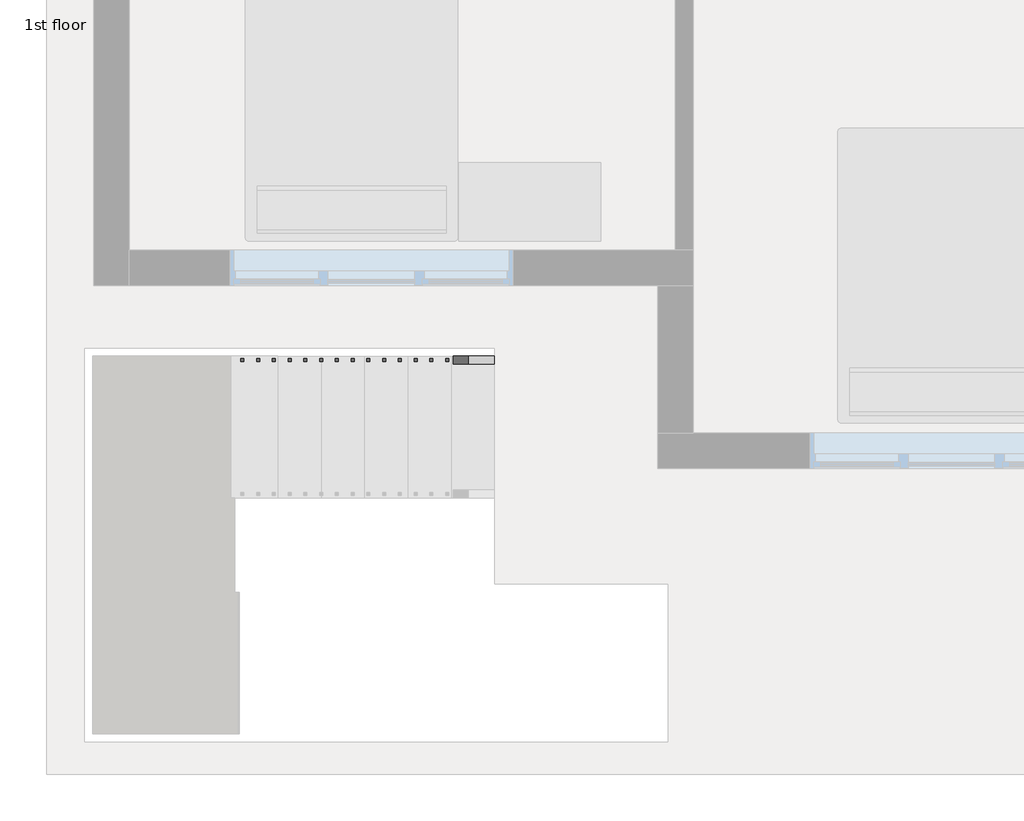
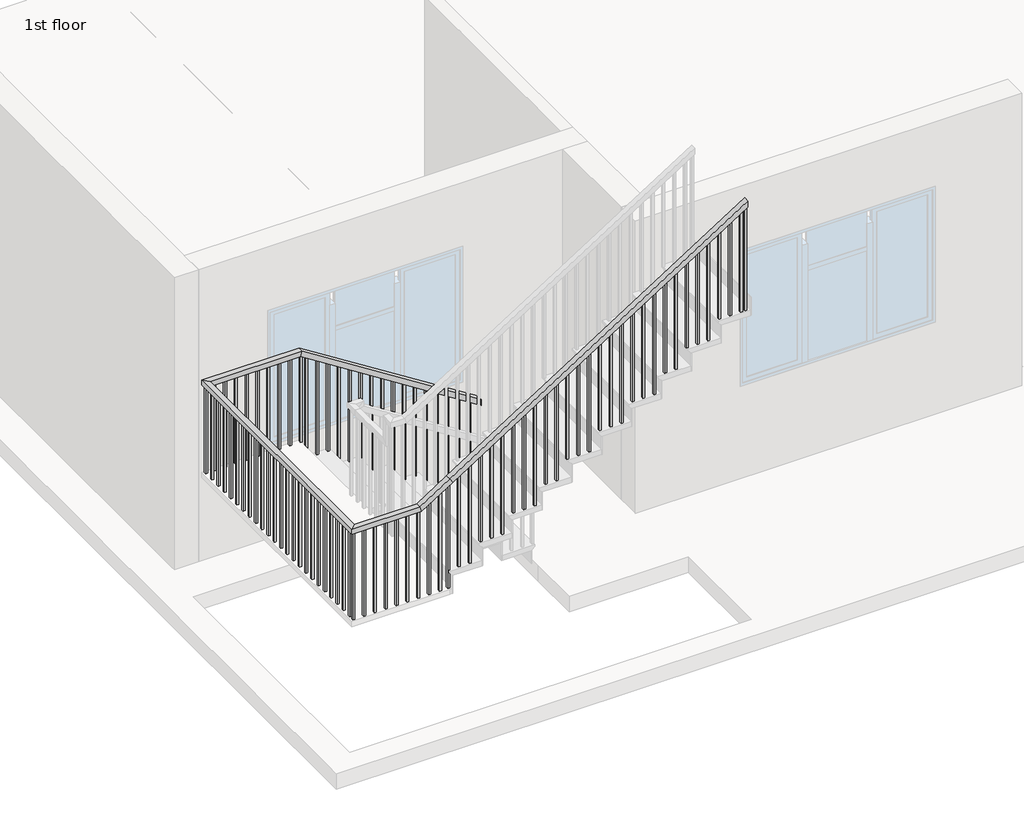
# One storey, part 3 of 4: 1 railing.
"""IFC4 building model written with IfcOpenShell, lengths in millimetres."""

from ifc_helpers import new_model, si_unit, frame, origin, place, context, project, spatial, polyline, outline, extrude, faceted_brep, element, save

model = new_model("IFC4")

# Units and contexts
model_context = context("Model", 3, world=origin())
ifc_project = project(units=[si_unit("LENGTHUNIT", "METRE", prefix="MILLI")], contexts=[model_context])

# Site, building, storey
site = spatial("IfcSite", under=ifc_project)
building = spatial("IfcBuilding", under=site)
storey = spatial("IfcBuildingStorey", under=building, Name="1st floor", Elevation=3810.0)

# Railing
placement = place(None, origin())
element("IfcRailing", 1, ObjectType="Handrail - Rectangular", at=placement, inside=storey, context=model_context, shape_type="SolidModel", body=[
    faceted_brep([(-6576.0763529, -1102.4338022, 4902.2), (-6576.0763529, -1102.4338022, 4841.986276), (-6576.0763529, -1051.6338022, 4841.986276), (-6576.0763529, -1051.6338022, 4902.2), (-8252.4763529, -1102.4338022, 5969.0), (-8267.2693478, -1102.4338022, 5918.2), (-8267.2693478, -1051.6338022, 5918.2), (-8252.4763529, -1051.6338022, 5969.0), (-9116.0763529, -1102.4338022, 5969.0), (-9116.0763529, -1102.4338022, 5918.2), (-9166.8763529, -1051.6338022, 5918.2), (-9166.8763529, -1051.6338022, 5969.0), (-9116.0763529, -3439.2338022, 5969.0), (-9116.0763529, -3439.2338022, 5918.2), (-9166.8763529, -3490.0338022, 5918.2), (-9166.8763529, -3490.0338022, 5969.0), (-8531.8763529, -3439.2338022, 5969.0), (-8517.083358, -3439.2338022, 5918.2), (-8517.083358, -3490.0338022, 5918.2), (-8531.8763529, -3490.0338022, 5969.0), (-8252.4763529, -3439.2338022, 6146.8), (-8225.2030779, -3439.2338022, 6103.9419964), (-8225.2030779, -3490.0338022, 6103.9419964), (-8252.4763529, -3490.0338022, 6146.8), (-5458.4763529, -3439.2338022, 7924.8), (-5458.4763529, -3490.0338022, 7924.8), (-5458.4763529, -3490.0338022, 7864.586276), (-5458.4763529, -3439.2338022, 7864.586276)], [[[0, 1, 2, 3]], [[1, 0, 4, 5]], [[2, 1, 5, 6]], [[3, 2, 6, 7]], [[0, 3, 7, 4]], [[5, 4, 8, 9]], [[6, 5, 9, 10]], [[7, 6, 10, 11]], [[4, 7, 11, 8]], [[9, 8, 12, 13]], [[10, 9, 13, 14]], [[11, 10, 14, 15]], [[8, 11, 15, 12]], [[13, 12, 16, 17]], [[14, 13, 17, 18]], [[15, 14, 18, 19]], [[12, 15, 19, 16]], [[17, 16, 20, 21]], [[18, 17, 21, 22]], [[19, 18, 22, 23]], [[16, 19, 23, 20]], [[24, 25, 26, 27]], [[21, 20, 24, 27]], [[22, 21, 27, 26]], [[23, 22, 26, 25]], [[20, 23, 25, 24]]]),
    extrude(outline(polyline([(7838.3203669, -5499.7513529), (7826.1976396, -5518.8013529), (6832.6, -5518.8013529), (6832.6, -5499.7513529), (7838.3203669, -5499.7513529)])), frame((0.0, -3474.1588022, 0.0), z_axis=(0.0, 1.0, 0.0), x_axis=(0.0, 0.0, 1.0)), (0.0, 0.0, 1.0), 19.05),
    extrude(outline(polyline([(7773.6658214, -5601.3513529), (7761.5430941, -5620.4013529), (6832.6, -5620.4013529), (6832.6, -5601.3513529), (7773.6658214, -5601.3513529)])), frame((0.0, -3474.1588022, 0.0), z_axis=(0.0, 1.0, 0.0), x_axis=(0.0, 0.0, 1.0)), (0.0, 0.0, 1.0), 19.05),
    extrude(outline(polyline([(7709.011276, -5702.9513529), (7696.8885487, -5722.0013529), (6832.6, -5722.0013529), (6832.6, -5702.9513529), (7709.011276, -5702.9513529)])), frame((0.0, -3474.1588022, 0.0), z_axis=(0.0, 1.0, 0.0), x_axis=(0.0, 0.0, 1.0)), (0.0, 0.0, 1.0), 19.05),
    extrude(outline(polyline([(7644.3567305, -5804.5513529), (7632.2340032, -5823.6013529), (6654.8, -5823.6013529), (6654.8, -5804.5513529), (7644.3567305, -5804.5513529)])), frame((0.0, -3474.1588022, 0.0), z_axis=(0.0, 1.0, 0.0), x_axis=(0.0, 0.0, 1.0)), (0.0, 0.0, 1.0), 19.05),
    extrude(outline(polyline([(7579.7021851, -5906.1513529), (7567.5794578, -5925.2013529), (6654.8, -5925.2013529), (6654.8, -5906.1513529), (7579.7021851, -5906.1513529)])), frame((0.0, -3474.1588022, 0.0), z_axis=(0.0, 1.0, 0.0), x_axis=(0.0, 0.0, 1.0)), (0.0, 0.0, 1.0), 19.05),
    extrude(outline(polyline([(7515.0476396, -6007.7513529), (7502.9249123, -6026.8013529), (6654.8, -6026.8013529), (6654.8, -6007.7513529), (7515.0476396, -6007.7513529)])), frame((0.0, -3474.1588022, 0.0), z_axis=(0.0, 1.0, 0.0), x_axis=(0.0, 0.0, 1.0)), (0.0, 0.0, 1.0), 19.05),
    extrude(outline(polyline([(7450.3930941, -6109.3513529), (7438.2703669, -6128.4013529), (6477.0, -6128.4013529), (6477.0, -6109.3513529), (7450.3930941, -6109.3513529)])), frame((0.0, -3474.1588022, 0.0), z_axis=(0.0, 1.0, 0.0), x_axis=(0.0, 0.0, 1.0)), (0.0, 0.0, 1.0), 19.05),
    extrude(outline(polyline([(7385.7385487, -6210.9513529), (7373.6158214, -6230.0013529), (6477.0, -6230.0013529), (6477.0, -6210.9513529), (7385.7385487, -6210.9513529)])), frame((0.0, -3474.1588022, 0.0), z_axis=(0.0, 1.0, 0.0), x_axis=(0.0, 0.0, 1.0)), (0.0, 0.0, 1.0), 19.05),
    extrude(outline(polyline([(7321.0840032, -6312.5513529), (7308.961276, -6331.6013529), (6299.2, -6331.6013529), (6299.2, -6312.5513529), (7321.0840032, -6312.5513529)])), frame((0.0, -3474.1588022, 0.0), z_axis=(0.0, 1.0, 0.0), x_axis=(0.0, 0.0, 1.0)), (0.0, 0.0, 1.0), 19.05),
    extrude(outline(polyline([(7256.4294578, -6414.1513529), (7244.3067305, -6433.2013529), (6299.2, -6433.2013529), (6299.2, -6414.1513529), (7256.4294578, -6414.1513529)])), frame((0.0, -3474.1588022, 0.0), z_axis=(0.0, 1.0, 0.0), x_axis=(0.0, 0.0, 1.0)), (0.0, 0.0, 1.0), 19.05),
    extrude(outline(polyline([(7191.7749123, -6515.7513529), (7179.6521851, -6534.8013529), (6299.2, -6534.8013529), (6299.2, -6515.7513529), (7191.7749123, -6515.7513529)])), frame((0.0, -3474.1588022, 0.0), z_axis=(0.0, 1.0, 0.0), x_axis=(0.0, 0.0, 1.0)), (0.0, 0.0, 1.0), 19.05),
    extrude(outline(polyline([(7127.1203669, -6617.3513529), (7114.9976396, -6636.4013529), (6121.4, -6636.4013529), (6121.4, -6617.3513529), (7127.1203669, -6617.3513529)])), frame((0.0, -3474.1588022, 0.0), z_axis=(0.0, 1.0, 0.0), x_axis=(0.0, 0.0, 1.0)), (0.0, 0.0, 1.0), 19.05),
    extrude(outline(polyline([(7062.4658214, -6718.9513529), (7050.3430941, -6738.0013529), (6121.4, -6738.0013529), (6121.4, -6718.9513529), (7062.4658214, -6718.9513529)])), frame((0.0, -3474.1588022, 0.0), z_axis=(0.0, 1.0, 0.0), x_axis=(0.0, 0.0, 1.0)), (0.0, 0.0, 1.0), 19.05),
    extrude(outline(polyline([(6997.811276, -6820.5513529), (6985.6885487, -6839.6013529), (6121.4, -6839.6013529), (6121.4, -6820.5513529), (6997.811276, -6820.5513529)])), frame((0.0, -3474.1588022, 0.0), z_axis=(0.0, 1.0, 0.0), x_axis=(0.0, 0.0, 1.0)), (0.0, 0.0, 1.0), 19.05),
    extrude(outline(polyline([(6933.1567305, -6922.1513529), (6921.0340032, -6941.2013529), (5943.6, -6941.2013529), (5943.6, -6922.1513529), (6933.1567305, -6922.1513529)])), frame((0.0, -3474.1588022, 0.0), z_axis=(0.0, 1.0, 0.0), x_axis=(0.0, 0.0, 1.0)), (0.0, 0.0, 1.0), 19.05),
    extrude(outline(polyline([(6868.5021851, -7023.7513529), (6856.3794578, -7042.8013529), (5943.6, -7042.8013529), (5943.6, -7023.7513529), (6868.5021851, -7023.7513529)])), frame((0.0, -3474.1588022, 0.0), z_axis=(0.0, 1.0, 0.0), x_axis=(0.0, 0.0, 1.0)), (0.0, 0.0, 1.0), 19.05),
    extrude(outline(polyline([(6803.8476396, -7125.3513529), (6791.7249123, -7144.4013529), (5943.6, -7144.4013529), (5943.6, -7125.3513529), (6803.8476396, -7125.3513529)])), frame((0.0, -3474.1588022, 0.0), z_axis=(0.0, 1.0, 0.0), x_axis=(0.0, 0.0, 1.0)), (0.0, 0.0, 1.0), 19.05),
    extrude(outline(polyline([(6739.1930941, -7226.9513529), (6727.0703669, -7246.0013529), (5765.8, -7246.0013529), (5765.8, -7226.9513529), (6739.1930941, -7226.9513529)])), frame((0.0, -3474.1588022, 0.0), z_axis=(0.0, 1.0, 0.0), x_axis=(0.0, 0.0, 1.0)), (0.0, 0.0, 1.0), 19.05),
    extrude(outline(polyline([(6674.5385487, -7328.5513529), (6662.4158214, -7347.6013529), (5765.8, -7347.6013529), (5765.8, -7328.5513529), (6674.5385487, -7328.5513529)])), frame((0.0, -3474.1588022, 0.0), z_axis=(0.0, 1.0, 0.0), x_axis=(0.0, 0.0, 1.0)), (0.0, 0.0, 1.0), 19.05),
    extrude(outline(polyline([(6609.8840032, -7430.1513529), (6597.761276, -7449.2013529), (5588.0, -7449.2013529), (5588.0, -7430.1513529), (6609.8840032, -7430.1513529)])), frame((0.0, -3474.1588022, 0.0), z_axis=(0.0, 1.0, 0.0), x_axis=(0.0, 0.0, 1.0)), (0.0, 0.0, 1.0), 19.05),
    extrude(outline(polyline([(6545.2294578, -7531.7513529), (6533.1067305, -7550.8013529), (5588.0, -7550.8013529), (5588.0, -7531.7513529), (6545.2294578, -7531.7513529)])), frame((0.0, -3474.1588022, 0.0), z_axis=(0.0, 1.0, 0.0), x_axis=(0.0, 0.0, 1.0)), (0.0, 0.0, 1.0), 19.05),
    extrude(outline(polyline([(6480.5749123, -7633.3513529), (6468.4521851, -7652.4013529), (5588.0, -7652.4013529), (5588.0, -7633.3513529), (6480.5749123, -7633.3513529)])), frame((0.0, -3474.1588022, 0.0), z_axis=(0.0, 1.0, 0.0), x_axis=(0.0, 0.0, 1.0)), (0.0, 0.0, 1.0), 19.05),
    extrude(outline(polyline([(6415.9203669, -7734.9513529), (6403.7976396, -7754.0013529), (5410.2, -7754.0013529), (5410.2, -7734.9513529), (6415.9203669, -7734.9513529)])), frame((0.0, -3474.1588022, 0.0), z_axis=(0.0, 1.0, 0.0), x_axis=(0.0, 0.0, 1.0)), (0.0, 0.0, 1.0), 19.05),
    extrude(outline(polyline([(6351.2658214, -7836.5513529), (6339.1430941, -7855.6013529), (5410.2, -7855.6013529), (5410.2, -7836.5513529), (6351.2658214, -7836.5513529)])), frame((0.0, -3474.1588022, 0.0), z_axis=(0.0, 1.0, 0.0), x_axis=(0.0, 0.0, 1.0)), (0.0, 0.0, 1.0), 19.05),
    extrude(outline(polyline([(6286.611276, -7938.1513529), (6274.4885487, -7957.2013529), (5410.2, -7957.2013529), (5410.2, -7938.1513529), (6286.611276, -7938.1513529)])), frame((0.0, -3474.1588022, 0.0), z_axis=(0.0, 1.0, 0.0), x_axis=(0.0, 0.0, 1.0)), (0.0, 0.0, 1.0), 19.05),
    extrude(outline(polyline([(6221.9567305, -8039.7513529), (6209.8340032, -8058.8013529), (5232.4, -8058.8013529), (5232.4, -8039.7513529), (6221.9567305, -8039.7513529)])), frame((0.0, -3474.1588022, 0.0), z_axis=(0.0, 1.0, 0.0), x_axis=(0.0, 0.0, 1.0)), (0.0, 0.0, 1.0), 19.05),
    extrude(outline(polyline([(6157.3021851, -8141.3513529), (6145.1794578, -8160.4013529), (5232.4, -8160.4013529), (5232.4, -8141.3513529), (6157.3021851, -8141.3513529)])), frame((0.0, -3474.1588022, 0.0), z_axis=(0.0, 1.0, 0.0), x_axis=(0.0, 0.0, 1.0)), (0.0, 0.0, 1.0), 19.05),
    extrude(outline(polyline([(6044.1567305, -8319.1513529), (6032.0340032, -8338.2013529), (5054.6, -8338.2013529), (5054.6, -8319.1513529), (6044.1567305, -8319.1513529)])), frame((0.0, -3474.1588022, 0.0), z_axis=(0.0, 1.0, 0.0), x_axis=(0.0, 0.0, 1.0)), (0.0, 0.0, 1.0), 19.05),
    extrude(outline(polyline([(5979.5021851, -8420.7513529), (5967.3794578, -8439.8013529), (5054.6, -8439.8013529), (5054.6, -8420.7513529), (5979.5021851, -8420.7513529)])), frame((0.0, -3474.1588022, 0.0), z_axis=(0.0, 1.0, 0.0), x_axis=(0.0, 0.0, 1.0)), (0.0, 0.0, 1.0), 19.05),
    extrude(outline(polyline([(-8541.4013529, -3474.1588022), (-8541.4013529, -3455.1088022), (-8522.3513529, -3455.1088022), (-8522.3513529, -3474.1588022), (-8541.4013529, -3474.1588022)])), frame((0.0, 0.0, 5054.6), z_axis=(0.0, 0.0, 1.0), x_axis=(1.0, 0.0, 0.0)), (0.0, 0.0, 1.0), 863.6),
    extrude(outline(polyline([(-8643.0013529, -3474.1588022), (-8643.0013529, -3455.1088022), (-8623.9513529, -3455.1088022), (-8623.9513529, -3474.1588022), (-8643.0013529, -3474.1588022)])), frame((0.0, 0.0, 5054.6), z_axis=(0.0, 0.0, 1.0), x_axis=(1.0, 0.0, 0.0)), (0.0, 0.0, 1.0), 863.6),
    extrude(outline(polyline([(-8744.6013529, -3474.1588022), (-8744.6013529, -3455.1088022), (-8725.5513529, -3455.1088022), (-8725.5513529, -3474.1588022), (-8744.6013529, -3474.1588022)])), frame((0.0, 0.0, 5054.6), z_axis=(0.0, 0.0, 1.0), x_axis=(1.0, 0.0, 0.0)), (0.0, 0.0, 1.0), 863.6),
    extrude(outline(polyline([(-8846.2013529, -3474.1588022), (-8846.2013529, -3455.1088022), (-8827.1513529, -3455.1088022), (-8827.1513529, -3474.1588022), (-8846.2013529, -3474.1588022)])), frame((0.0, 0.0, 5054.6), z_axis=(0.0, 0.0, 1.0), x_axis=(1.0, 0.0, 0.0)), (0.0, 0.0, 1.0), 863.6),
    extrude(outline(polyline([(-8947.8013529, -3474.1588022), (-8947.8013529, -3455.1088022), (-8928.7513529, -3455.1088022), (-8928.7513529, -3474.1588022), (-8947.8013529, -3474.1588022)])), frame((0.0, 0.0, 5054.6), z_axis=(0.0, 0.0, 1.0), x_axis=(1.0, 0.0, 0.0)), (0.0, 0.0, 1.0), 863.6),
    extrude(outline(polyline([(-9049.4013529, -3474.1588022), (-9049.4013529, -3455.1088022), (-9030.3513529, -3455.1088022), (-9030.3513529, -3474.1588022), (-9049.4013529, -3474.1588022)])), frame((0.0, 0.0, 5054.6), z_axis=(0.0, 0.0, 1.0), x_axis=(1.0, 0.0, 0.0)), (0.0, 0.0, 1.0), 863.6),
    extrude(outline(polyline([(-9151.0013529, -3404.3088022), (-9131.9513529, -3404.3088022), (-9131.9513529, -3423.3588022), (-9151.0013529, -3423.3588022), (-9151.0013529, -3404.3088022)])), frame((0.0, 0.0, 5054.6), z_axis=(0.0, 0.0, 1.0), x_axis=(1.0, 0.0, 0.0)), (0.0, 0.0, 1.0), 863.6),
    extrude(outline(polyline([(-9151.0013529, -3302.7088022), (-9131.9513529, -3302.7088022), (-9131.9513529, -3321.7588022), (-9151.0013529, -3321.7588022), (-9151.0013529, -3302.7088022)])), frame((0.0, 0.0, 5054.6), z_axis=(0.0, 0.0, 1.0), x_axis=(1.0, 0.0, 0.0)), (0.0, 0.0, 1.0), 863.6),
    extrude(outline(polyline([(-9151.0013529, -3201.1088022), (-9131.9513529, -3201.1088022), (-9131.9513529, -3220.1588022), (-9151.0013529, -3220.1588022), (-9151.0013529, -3201.1088022)])), frame((0.0, 0.0, 5054.6), z_axis=(0.0, 0.0, 1.0), x_axis=(1.0, 0.0, 0.0)), (0.0, 0.0, 1.0), 863.6),
    extrude(outline(polyline([(-9151.0013529, -3099.5088022), (-9131.9513529, -3099.5088022), (-9131.9513529, -3118.5588022), (-9151.0013529, -3118.5588022), (-9151.0013529, -3099.5088022)])), frame((0.0, 0.0, 5054.6), z_axis=(0.0, 0.0, 1.0), x_axis=(1.0, 0.0, 0.0)), (0.0, 0.0, 1.0), 863.6),
    extrude(outline(polyline([(-9151.0013529, -2997.9088022), (-9131.9513529, -2997.9088022), (-9131.9513529, -3016.9588022), (-9151.0013529, -3016.9588022), (-9151.0013529, -2997.9088022)])), frame((0.0, 0.0, 5054.6), z_axis=(0.0, 0.0, 1.0), x_axis=(1.0, 0.0, 0.0)), (0.0, 0.0, 1.0), 863.6),
    extrude(outline(polyline([(-9151.0013529, -2896.3088022), (-9131.9513529, -2896.3088022), (-9131.9513529, -2915.3588022), (-9151.0013529, -2915.3588022), (-9151.0013529, -2896.3088022)])), frame((0.0, 0.0, 5054.6), z_axis=(0.0, 0.0, 1.0), x_axis=(1.0, 0.0, 0.0)), (0.0, 0.0, 1.0), 863.6),
    extrude(outline(polyline([(-9151.0013529, -2794.7088022), (-9131.9513529, -2794.7088022), (-9131.9513529, -2813.7588022), (-9151.0013529, -2813.7588022), (-9151.0013529, -2794.7088022)])), frame((0.0, 0.0, 5054.6), z_axis=(0.0, 0.0, 1.0), x_axis=(1.0, 0.0, 0.0)), (0.0, 0.0, 1.0), 863.6),
    extrude(outline(polyline([(-9151.0013529, -2693.1088022), (-9131.9513529, -2693.1088022), (-9131.9513529, -2712.1588022), (-9151.0013529, -2712.1588022), (-9151.0013529, -2693.1088022)])), frame((0.0, 0.0, 5054.6), z_axis=(0.0, 0.0, 1.0), x_axis=(1.0, 0.0, 0.0)), (0.0, 0.0, 1.0), 863.6),
    extrude(outline(polyline([(-9151.0013529, -2591.5088022), (-9131.9513529, -2591.5088022), (-9131.9513529, -2610.5588022), (-9151.0013529, -2610.5588022), (-9151.0013529, -2591.5088022)])), frame((0.0, 0.0, 5054.6), z_axis=(0.0, 0.0, 1.0), x_axis=(1.0, 0.0, 0.0)), (0.0, 0.0, 1.0), 863.6),
    extrude(outline(polyline([(-9151.0013529, -2489.9088022), (-9131.9513529, -2489.9088022), (-9131.9513529, -2508.9588022), (-9151.0013529, -2508.9588022), (-9151.0013529, -2489.9088022)])), frame((0.0, 0.0, 5054.6), z_axis=(0.0, 0.0, 1.0), x_axis=(1.0, 0.0, 0.0)), (0.0, 0.0, 1.0), 863.6),
    extrude(outline(polyline([(-9151.0013529, -2388.3088022), (-9131.9513529, -2388.3088022), (-9131.9513529, -2407.3588022), (-9151.0013529, -2407.3588022), (-9151.0013529, -2388.3088022)])), frame((0.0, 0.0, 5054.6), z_axis=(0.0, 0.0, 1.0), x_axis=(1.0, 0.0, 0.0)), (0.0, 0.0, 1.0), 863.6),
    extrude(outline(polyline([(-9151.0013529, -2286.7088022), (-9131.9513529, -2286.7088022), (-9131.9513529, -2305.7588022), (-9151.0013529, -2305.7588022), (-9151.0013529, -2286.7088022)])), frame((0.0, 0.0, 5054.6), z_axis=(0.0, 0.0, 1.0), x_axis=(1.0, 0.0, 0.0)), (0.0, 0.0, 1.0), 863.6),
    extrude(outline(polyline([(-9151.0013529, -2185.1088022), (-9131.9513529, -2185.1088022), (-9131.9513529, -2204.1588022), (-9151.0013529, -2204.1588022), (-9151.0013529, -2185.1088022)])), frame((0.0, 0.0, 5054.6), z_axis=(0.0, 0.0, 1.0), x_axis=(1.0, 0.0, 0.0)), (0.0, 0.0, 1.0), 863.6),
    extrude(outline(polyline([(-9151.0013529, -2083.5088022), (-9131.9513529, -2083.5088022), (-9131.9513529, -2102.5588022), (-9151.0013529, -2102.5588022), (-9151.0013529, -2083.5088022)])), frame((0.0, 0.0, 5054.6), z_axis=(0.0, 0.0, 1.0), x_axis=(1.0, 0.0, 0.0)), (0.0, 0.0, 1.0), 863.6),
    extrude(outline(polyline([(-9151.0013529, -1981.9088022), (-9131.9513529, -1981.9088022), (-9131.9513529, -2000.9588022), (-9151.0013529, -2000.9588022), (-9151.0013529, -1981.9088022)])), frame((0.0, 0.0, 5054.6), z_axis=(0.0, 0.0, 1.0), x_axis=(1.0, 0.0, 0.0)), (0.0, 0.0, 1.0), 863.6),
    extrude(outline(polyline([(-9151.0013529, -1880.3088022), (-9131.9513529, -1880.3088022), (-9131.9513529, -1899.3588022), (-9151.0013529, -1899.3588022), (-9151.0013529, -1880.3088022)])), frame((0.0, 0.0, 5054.6), z_axis=(0.0, 0.0, 1.0), x_axis=(1.0, 0.0, 0.0)), (0.0, 0.0, 1.0), 863.6),
    extrude(outline(polyline([(-9151.0013529, -1778.7088022), (-9131.9513529, -1778.7088022), (-9131.9513529, -1797.7588022), (-9151.0013529, -1797.7588022), (-9151.0013529, -1778.7088022)])), frame((0.0, 0.0, 5054.6), z_axis=(0.0, 0.0, 1.0), x_axis=(1.0, 0.0, 0.0)), (0.0, 0.0, 1.0), 863.6),
    extrude(outline(polyline([(-9151.0013529, -1677.1088022), (-9131.9513529, -1677.1088022), (-9131.9513529, -1696.1588022), (-9151.0013529, -1696.1588022), (-9151.0013529, -1677.1088022)])), frame((0.0, 0.0, 5054.6), z_axis=(0.0, 0.0, 1.0), x_axis=(1.0, 0.0, 0.0)), (0.0, 0.0, 1.0), 863.6),
    extrude(outline(polyline([(-9151.0013529, -1575.5088022), (-9131.9513529, -1575.5088022), (-9131.9513529, -1594.5588022), (-9151.0013529, -1594.5588022), (-9151.0013529, -1575.5088022)])), frame((0.0, 0.0, 5054.6), z_axis=(0.0, 0.0, 1.0), x_axis=(1.0, 0.0, 0.0)), (0.0, 0.0, 1.0), 863.6),
    extrude(outline(polyline([(-9151.0013529, -1473.9088022), (-9131.9513529, -1473.9088022), (-9131.9513529, -1492.9588022), (-9151.0013529, -1492.9588022), (-9151.0013529, -1473.9088022)])), frame((0.0, 0.0, 5054.6), z_axis=(0.0, 0.0, 1.0), x_axis=(1.0, 0.0, 0.0)), (0.0, 0.0, 1.0), 863.6),
    extrude(outline(polyline([(-9151.0013529, -1372.3088022), (-9131.9513529, -1372.3088022), (-9131.9513529, -1391.3588022), (-9151.0013529, -1391.3588022), (-9151.0013529, -1372.3088022)])), frame((0.0, 0.0, 5054.6), z_axis=(0.0, 0.0, 1.0), x_axis=(1.0, 0.0, 0.0)), (0.0, 0.0, 1.0), 863.6),
    extrude(outline(polyline([(-9151.0013529, -1270.7088022), (-9131.9513529, -1270.7088022), (-9131.9513529, -1289.7588022), (-9151.0013529, -1289.7588022), (-9151.0013529, -1270.7088022)])), frame((0.0, 0.0, 5054.6), z_axis=(0.0, 0.0, 1.0), x_axis=(1.0, 0.0, 0.0)), (0.0, 0.0, 1.0), 863.6),
    extrude(outline(polyline([(-9151.0013529, -1169.1088022), (-9131.9513529, -1169.1088022), (-9131.9513529, -1188.1588022), (-9151.0013529, -1188.1588022), (-9151.0013529, -1169.1088022)])), frame((0.0, 0.0, 5054.6), z_axis=(0.0, 0.0, 1.0), x_axis=(1.0, 0.0, 0.0)), (0.0, 0.0, 1.0), 863.6),
    extrude(outline(polyline([(-9055.7513529, -1067.5088022), (-9055.7513529, -1086.5588022), (-9074.8013529, -1086.5588022), (-9074.8013529, -1067.5088022), (-9055.7513529, -1067.5088022)])), frame((0.0, 0.0, 5054.6), z_axis=(0.0, 0.0, 1.0), x_axis=(1.0, 0.0, 0.0)), (0.0, 0.0, 1.0), 863.6),
    extrude(outline(polyline([(-8954.1513529, -1067.5088022), (-8954.1513529, -1086.5588022), (-8973.2013529, -1086.5588022), (-8973.2013529, -1067.5088022), (-8954.1513529, -1067.5088022)])), frame((0.0, 0.0, 5054.6), z_axis=(0.0, 0.0, 1.0), x_axis=(1.0, 0.0, 0.0)), (0.0, 0.0, 1.0), 863.6),
    extrude(outline(polyline([(-8852.5513529, -1067.5088022), (-8852.5513529, -1086.5588022), (-8871.6013529, -1086.5588022), (-8871.6013529, -1067.5088022), (-8852.5513529, -1067.5088022)])), frame((0.0, 0.0, 5054.6), z_axis=(0.0, 0.0, 1.0), x_axis=(1.0, 0.0, 0.0)), (0.0, 0.0, 1.0), 863.6),
    extrude(outline(polyline([(-8750.9513529, -1067.5088022), (-8750.9513529, -1086.5588022), (-8770.0013529, -1086.5588022), (-8770.0013529, -1067.5088022), (-8750.9513529, -1067.5088022)])), frame((0.0, 0.0, 5054.6), z_axis=(0.0, 0.0, 1.0), x_axis=(1.0, 0.0, 0.0)), (0.0, 0.0, 1.0), 863.6),
    extrude(outline(polyline([(-8649.3513529, -1067.5088022), (-8649.3513529, -1086.5588022), (-8668.4013529, -1086.5588022), (-8668.4013529, -1067.5088022), (-8649.3513529, -1067.5088022)])), frame((0.0, 0.0, 5054.6), z_axis=(0.0, 0.0, 1.0), x_axis=(1.0, 0.0, 0.0)), (0.0, 0.0, 1.0), 863.6),
    extrude(outline(polyline([(-8547.7513529, -1067.5088022), (-8547.7513529, -1086.5588022), (-8566.8013529, -1086.5588022), (-8566.8013529, -1067.5088022), (-8547.7513529, -1067.5088022)])), frame((0.0, 0.0, 5054.6), z_axis=(0.0, 0.0, 1.0), x_axis=(1.0, 0.0, 0.0)), (0.0, 0.0, 1.0), 863.6),
    extrude(outline(polyline([(-8446.1513529, -1067.5088022), (-8446.1513529, -1086.5588022), (-8465.2013529, -1086.5588022), (-8465.2013529, -1067.5088022), (-8446.1513529, -1067.5088022)])), frame((0.0, 0.0, 5054.6), z_axis=(0.0, 0.0, 1.0), x_axis=(1.0, 0.0, 0.0)), (0.0, 0.0, 1.0), 863.6),
    extrude(outline(polyline([(-8344.5513529, -1067.5088022), (-8344.5513529, -1086.5588022), (-8363.6013529, -1086.5588022), (-8363.6013529, -1067.5088022), (-8344.5513529, -1067.5088022)])), frame((0.0, 0.0, 5054.6), z_axis=(0.0, 0.0, 1.0), x_axis=(1.0, 0.0, 0.0)), (0.0, 0.0, 1.0), 863.6),
    extrude(outline(polyline([(5870.3976396, -8192.1513529), (5882.5203669, -8211.2013529), (4876.8, -8211.2013529), (4876.8, -8192.1513529), (5870.3976396, -8192.1513529)])), frame((0.0, -1086.5588022, 0.0), z_axis=(0.0, 1.0, 0.0), x_axis=(0.0, 0.0, 1.0)), (0.0, 0.0, 1.0), 19.05),
    extrude(outline(polyline([(5805.7430941, -8090.5513529), (5817.8658214, -8109.6013529), (4876.8, -8109.6013529), (4876.8, -8090.5513529), (5805.7430941, -8090.5513529)])), frame((0.0, -1086.5588022, 0.0), z_axis=(0.0, 1.0, 0.0), x_axis=(0.0, 0.0, 1.0)), (0.0, 0.0, 1.0), 19.05),
    extrude(outline(polyline([(5741.0885487, -7988.9513529), (5753.211276, -8008.0013529), (4876.8, -8008.0013529), (4876.8, -7988.9513529), (5741.0885487, -7988.9513529)])), frame((0.0, -1086.5588022, 0.0), z_axis=(0.0, 1.0, 0.0), x_axis=(0.0, 0.0, 1.0)), (0.0, 0.0, 1.0), 19.05),
    extrude(outline(polyline([(5676.4340032, -7887.3513529), (5688.5567305, -7906.4013529), (4699.0, -7906.4013529), (4699.0, -7887.3513529), (5676.4340032, -7887.3513529)])), frame((0.0, -1086.5588022, 0.0), z_axis=(0.0, 1.0, 0.0), x_axis=(0.0, 0.0, 1.0)), (0.0, 0.0, 1.0), 19.05),
    extrude(outline(polyline([(5611.7794578, -7785.7513529), (5623.9021851, -7804.8013529), (4699.0, -7804.8013529), (4699.0, -7785.7513529), (5611.7794578, -7785.7513529)])), frame((0.0, -1086.5588022, 0.0), z_axis=(0.0, 1.0, 0.0), x_axis=(0.0, 0.0, 1.0)), (0.0, 0.0, 1.0), 19.05),
    extrude(outline(polyline([(5547.1249123, -7684.1513529), (5559.2476396, -7703.2013529), (4699.0, -7703.2013529), (4699.0, -7684.1513529), (5547.1249123, -7684.1513529)])), frame((0.0, -1086.5588022, 0.0), z_axis=(0.0, 1.0, 0.0), x_axis=(0.0, 0.0, 1.0)), (0.0, 0.0, 1.0), 19.05),
    extrude(outline(polyline([(5482.4703669, -7582.5513529), (5494.5930941, -7601.6013529), (4521.2, -7601.6013529), (4521.2, -7582.5513529), (5482.4703669, -7582.5513529)])), frame((0.0, -1086.5588022, 0.0), z_axis=(0.0, 1.0, 0.0), x_axis=(0.0, 0.0, 1.0)), (0.0, 0.0, 1.0), 19.05),
    extrude(outline(polyline([(5417.8158214, -7480.9513529), (5429.9385487, -7500.0013529), (4521.2, -7500.0013529), (4521.2, -7480.9513529), (5417.8158214, -7480.9513529)])), frame((0.0, -1086.5588022, 0.0), z_axis=(0.0, 1.0, 0.0), x_axis=(0.0, 0.0, 1.0)), (0.0, 0.0, 1.0), 19.05),
    extrude(outline(polyline([(5353.161276, -7379.3513529), (5365.2840032, -7398.4013529), (4343.4, -7398.4013529), (4343.4, -7379.3513529), (5353.161276, -7379.3513529)])), frame((0.0, -1086.5588022, 0.0), z_axis=(0.0, 1.0, 0.0), x_axis=(0.0, 0.0, 1.0)), (0.0, 0.0, 1.0), 19.05),
    extrude(outline(polyline([(5288.5067305, -7277.7513529), (5300.6294578, -7296.8013529), (4343.4, -7296.8013529), (4343.4, -7277.7513529), (5288.5067305, -7277.7513529)])), frame((0.0, -1086.5588022, 0.0), z_axis=(0.0, 1.0, 0.0), x_axis=(0.0, 0.0, 1.0)), (0.0, 0.0, 1.0), 19.05),
    extrude(outline(polyline([(5223.8521851, -7176.1513529), (5235.9749123, -7195.2013529), (4343.4, -7195.2013529), (4343.4, -7176.1513529), (5223.8521851, -7176.1513529)])), frame((0.0, -1086.5588022, 0.0), z_axis=(0.0, 1.0, 0.0), x_axis=(0.0, 0.0, 1.0)), (0.0, 0.0, 1.0), 19.05),
    extrude(outline(polyline([(5159.1976396, -7074.5513529), (5171.3203669, -7093.6013529), (4165.6, -7093.6013529), (4165.6, -7074.5513529), (5159.1976396, -7074.5513529)])), frame((0.0, -1086.5588022, 0.0), z_axis=(0.0, 1.0, 0.0), x_axis=(0.0, 0.0, 1.0)), (0.0, 0.0, 1.0), 19.05),
    extrude(outline(polyline([(5094.5430941, -6972.9513529), (5106.6658214, -6992.0013529), (4165.6, -6992.0013529), (4165.6, -6972.9513529), (5094.5430941, -6972.9513529)])), frame((0.0, -1086.5588022, 0.0), z_axis=(0.0, 1.0, 0.0), x_axis=(0.0, 0.0, 1.0)), (0.0, 0.0, 1.0), 19.05),
    extrude(outline(polyline([(5029.8885487, -6871.3513529), (5042.011276, -6890.4013529), (4165.6, -6890.4013529), (4165.6, -6871.3513529), (5029.8885487, -6871.3513529)])), frame((0.0, -1086.5588022, 0.0), z_axis=(0.0, 1.0, 0.0), x_axis=(0.0, 0.0, 1.0)), (0.0, 0.0, 1.0), 19.05),
    extrude(outline(polyline([(4965.2340032, -6769.7513529), (4977.3567305, -6788.8013529), (3987.8, -6788.8013529), (3987.8, -6769.7513529), (4965.2340032, -6769.7513529)])), frame((0.0, -1086.5588022, 0.0), z_axis=(0.0, 1.0, 0.0), x_axis=(0.0, 0.0, 1.0)), (0.0, 0.0, 1.0), 19.05),
    extrude(outline(polyline([(4900.5794578, -6668.1513529), (4912.7021851, -6687.2013529), (3987.8, -6687.2013529), (3987.8, -6668.1513529), (4900.5794578, -6668.1513529)])), frame((0.0, -1086.5588022, 0.0), z_axis=(0.0, 1.0, 0.0), x_axis=(0.0, 0.0, 1.0)), (0.0, 0.0, 1.0), 19.05),
    extrude(outline(polyline([(6092.6476396, -8242.9513529), (6080.5249123, -8262.0013529), (5054.6, -8262.0013529), (5054.6, -8242.9513529), (6092.6476396, -8242.9513529)])), frame((0.0, -3474.1588022, 0.0), z_axis=(0.0, 1.0, 0.0), x_axis=(0.0, 0.0, 1.0)), (0.0, 0.0, 1.0), 19.05),
    extrude(outline(polyline([(-9151.0013529, -3455.1088022), (-9131.9513529, -3455.1088022), (-9131.9513529, -3474.1588022), (-9151.0013529, -3474.1588022), (-9151.0013529, -3455.1088022)])), frame((0.0, 0.0, 5054.6), z_axis=(0.0, 0.0, 1.0), x_axis=(1.0, 0.0, 0.0)), (0.0, 0.0, 1.0), 863.6),
    extrude(outline(polyline([(-9131.9513529, -1067.5088022), (-9131.9513529, -1086.5588022), (-9151.0013529, -1086.5588022), (-9151.0013529, -1067.5088022), (-9131.9513529, -1067.5088022)])), frame((0.0, 0.0, 5054.6), z_axis=(0.0, 0.0, 1.0), x_axis=(1.0, 0.0, 0.0)), (0.0, 0.0, 1.0), 863.6),
    extrude(outline(polyline([(5902.7249123, -8242.9513529), (5914.8476396, -8262.0013529), (5054.6, -8262.0013529), (5054.6, -8242.9513529), (5902.7249123, -8242.9513529)])), frame((0.0, -1086.5588022, 0.0), z_axis=(0.0, 1.0, 0.0), x_axis=(0.0, 0.0, 1.0)), (0.0, 0.0, 1.0), 19.05),
    extrude(outline(polyline([(7864.586276, -5458.4763529), (7852.4635487, -5477.5263529), (6832.6, -5477.5263529), (6832.6, -5458.4763529), (7864.586276, -5458.4763529)])), frame((0.0, -3474.1588022, 0.0), z_axis=(0.0, 1.0, 0.0), x_axis=(0.0, 0.0, 1.0)), (0.0, 0.0, 1.0), 19.05),
    extrude(outline(polyline([(4841.986276, -6576.0763529), (4854.1090032, -6595.1263529), (3987.8, -6595.1263529), (3987.8, -6576.0763529), (4841.986276, -6576.0763529)])), frame((0.0, -1086.5588022, 0.0), z_axis=(0.0, 1.0, 0.0), x_axis=(0.0, 0.0, 1.0)), (0.0, 0.0, 1.0), 19.05),
])

save(model, "model.ifc")

# Revit data of these elements
# Type "Handrail - Rectangular"
#   Assembly Code = "C2010400"
#   built-in parameter 1008612 = 0.0416667 (stored number, unit not read)
#   built-in parameter 1008611 = 0.0416667 (stored number, unit not read)
#   built-in parameter 1008609 = 0.333333 (stored number, unit not read)
#   built-in parameter 1008604 = 0.166667 (stored number, unit not read)
#   built-in parameter 1008603 = 0.166667 (stored number, unit not read)
#   Railing Height = 3' - 0"
#   built-in parameter 1008630 = 2
#   built-in parameter 1008610 = 2
#   built-in parameter 1008618 = Baluster - Square : 3/4"
# Element 1 (IfcRailing, "Handrail - Rectangular")
#   Phase Created = New Construction
